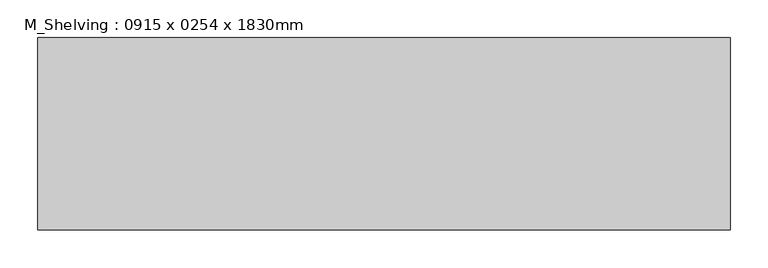
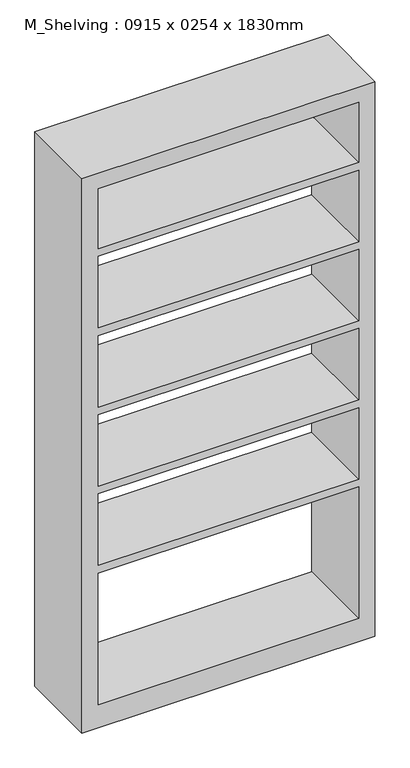
"""IFC4 building model written with IfcOpenShell, lengths in millimetres: furniture geometry, M_Shelving : 0915 x 0254 x 1830mm."""

from ifc_helpers import new_model, si_unit, frame, origin, place, context, project, spatial, polyline, outline, extrude, source, transform, mapped, element, save


def m_shelving_0915_x_0254_x_1830mm_1d5e155e(model_context):
    return source(origin(), model_context, "Body", "SweptSolid", [
        extrude(outline(polyline([(0.0, 457.5), (1830.0, 457.5), (1830.0, -457.5), (0.0, -457.5), (0.0, 457.5)]), holes=[polyline([(1779.2, 406.7), (1581.2714286, 406.7), (1581.2714286, -406.7), (1779.2, -406.7), (1779.2, 406.7)]), polyline([(76.2, 406.7), (76.2, -406.7), (510.1571429, -406.7), (510.1571429, 406.7), (76.2, 406.7)]), polyline([(1058.4142857, -406.7), (1294.4428571, -406.7), (1294.4428571, 406.7), (1058.4142857, 406.7), (1058.4142857, -406.7)]), polyline([(1555.8714286, 406.7), (1319.8428571, 406.7), (1319.8428571, -406.7), (1555.8714286, -406.7), (1555.8714286, 406.7)]), polyline([(1033.0142857, 406.7), (796.9857143, 406.7), (796.9857143, -406.7), (1033.0142857, -406.7), (1033.0142857, 406.7)]), polyline([(771.5857143, 406.7), (535.5571429, 406.7), (535.5571429, -406.7), (771.5857143, -406.7), (771.5857143, 406.7)])]), frame((0.0, -431.8, 0.0), z_axis=(0.0, 1.0, 0.0), x_axis=(0.0, 0.0, 1.0)), (0.0, 0.0, 1.0), 254.0),
    ])


if __name__ == "__main__":
    model = new_model("IFC4")
    model_context = context("Model", 3, world=origin())
    ifc_project = project(units=[si_unit("LENGTHUNIT", "METRE", prefix="MILLI")], contexts=[model_context])
    site = spatial("IfcSite", under=ifc_project)
    building = spatial("IfcBuilding", under=site)
    placement = place(None, origin())
    m_shelving_0915_x_0254_x_1830mm_shape = m_shelving_0915_x_0254_x_1830mm_1d5e155e(model_context)
    element("IfcFurniture", 1, ObjectType="M_Shelving : 0915 x 0254 x 1830mm", at=placement, inside=building, context=model_context, shape_type="MappedRepresentation", body=[
        mapped(m_shelving_0915_x_0254_x_1830mm_shape, transform((0.0, 0.0, 0.0), x_axis=(1.0, 0.0, 0.0), y_axis=(0.0, 1.0, 0.0), z_axis=(0.0, 0.0, 1.0))),
    ])
    save(model, "model.ifc")

# Revit data of these elements
# Type "M_Shelving : 0915 x 0254 x 1830mm"
#   Depth = 254 mm
#   Height = 1830 mm
#   Width = 915 mm
#   Material = Birch
#   Default Elevation = 0
# Element 1 (IfcFurniture, "M_Shelving : 0915 x 0254 x 1830mm")
#   Materials on its faces: "Birch"
# Materials
#   "Birch": class "Wood", colour RGB 224 178 126, transparency 0, Description = "Betula Alleghaniensis", Cost = 0
